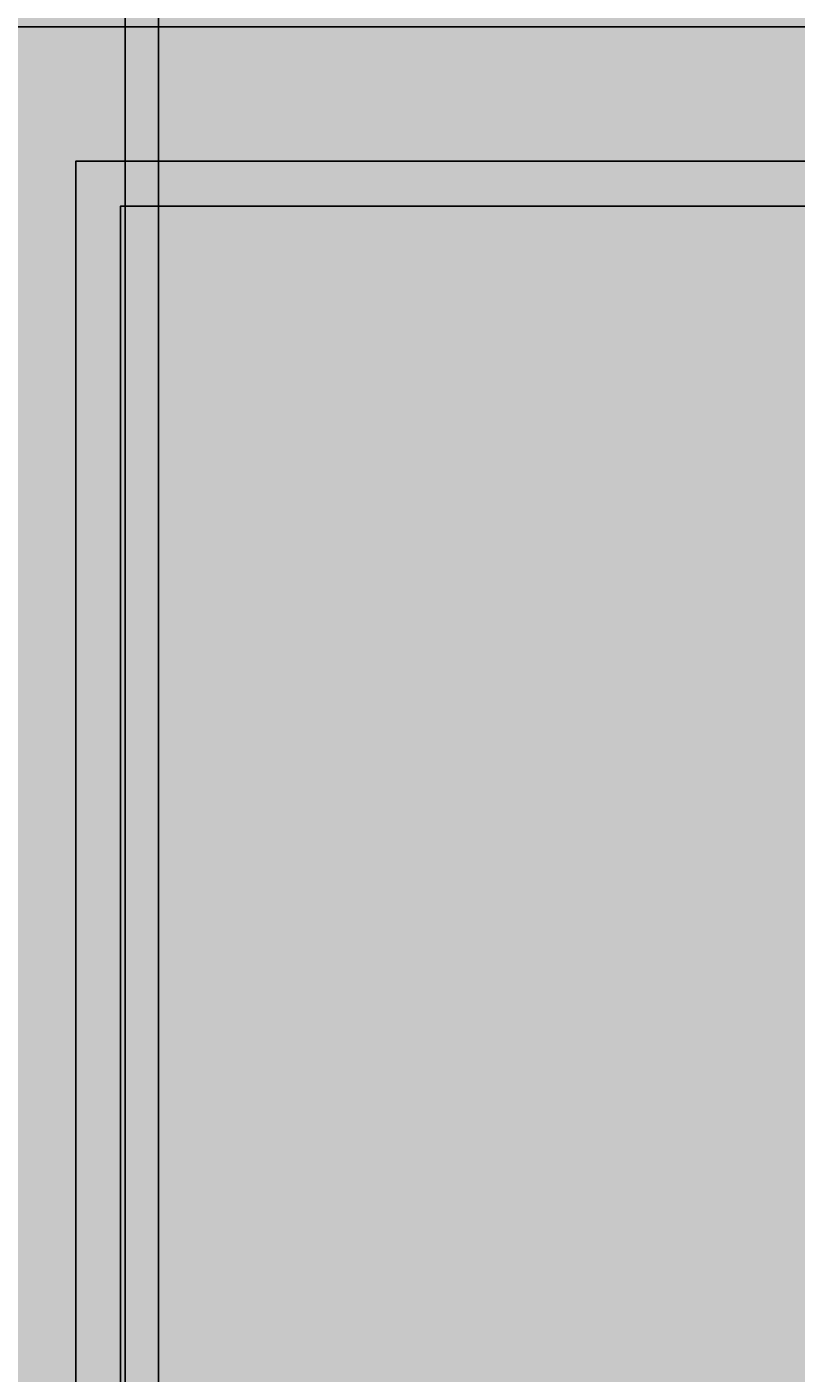
# Model space of a CAD drawing. Units: feet. Extents: x 2695 to 2912, y 795 to 1139.
# Tile 26 of 83: x 2808 to 2825, y 875 to 906. Entities that reach past the tile are written whole.
import ezdxf

# ---------------------------------------------------------------- set-up
doc = ezdxf.new("R2010")
doc.units = ezdxf.units.FT
for name, color, linetype, lineweight in [('A-ANNO-DIMS', 2, 'Continuous', 18), ('A-DOOR', 3, 'Continuous', 25), ('A-DOOR-PATT', 33, 'Continuous', 13), ('A-ELEV-PATT', 252, 'Continuous', 13)]:
    doc.layers.add(name, color=color, linetype=linetype, lineweight=lineweight)
doc.styles.get("Standard").update_dxf_attribs({"font": 'arial.ttf'})
doc.dimstyles.get("Standard").update_dxf_attribs({"dimtxt": 0.18, "dimasz": 0.18, "dimexe": 0.18, "dimexo": 0.0625, "dimgap": 0.09, "dimtad": 0, "dimtih": 1, "dimtoh": 1, "dimdec": 1, "dimzin": 0, "dimdsep": 46, "dimlunit": 3, "dimtxsty": 'Standard', "dimcen": 0.09, "dimadec": 0, "dimazin": 0, "dimtfac": 1, "dimtdec": 1, "dimtofl": 0, "dimtmove": 0, "dimatfit": 3, "dimfxl": 1, "dimtolj": 1, "dimtzin": 0, "dimarcsym": 0})

# ---------------------------------------------------------------- blocks, each defined once
blk = doc.blocks.new('*D14')
at = {"layer": 'A-ANNO-DIMS', "color": 0, "lineweight": -2, "transparency": 16777216}
for p, q in [((2838.439, 905.514), (2911.424, 905.514)), ((2911.244, 905.334), (2911.244, 890.368)), ((2911.244, 875.037), (2911.244, 890.004)), ((2758.214, 874.857), (2911.424, 874.857))]:
    blk.add_line(p, q, dxfattribs=at)
at = {"layer": 'A-ANNO-DIMS', "color": 0, "transparency": 16777216}
for points in [[(2911.214, 905.334), (2911.274, 905.334), (2911.244, 905.514)], [(2911.214, 875.037), (2911.274, 875.037), (2911.244, 874.857)]]:
    blk.add_solid(points, dxfattribs=at)
at = {"layer": 'Defpoints', "color": 0, "transparency": 16777216}
for p in [(2838.377, 905.514), (2911.244, 905.514), (2758.151, 874.857)]:
    blk.add_point(p, dxfattribs=at)
at = {"layer": 'A-ANNO-DIMS', "color": 0, "transparency": 16777216, "insert": (2911.244, 890.186), "char_height": 0.18, "attachment_point": 5}
blk.add_mtext('\\A1;30.66', dxfattribs=at)
blk = doc.blocks.new('*D52')
at = {"layer": 'A-ANNO-DIMS', "color": 0, "lineweight": -2, "transparency": 16777216}
for p, q in [((2810.041, 936.868), (2810.041, 794.976)), ((2810.789, 936.868), (2810.789, 794.976)), ((2809.861, 795.156), (2809.681, 795.156)), ((2810.969, 795.156), (2811.149, 795.156))]:
    blk.add_line(p, q, dxfattribs=at)
at = {"layer": 'A-ANNO-DIMS', "color": 0, "transparency": 16777216}
for points in [[(2809.861, 795.186), (2809.861, 795.126), (2810.041, 795.156)], [(2810.969, 795.186), (2810.969, 795.126), (2810.789, 795.156)]]:
    blk.add_solid(points, dxfattribs=at)
at = {"layer": 'Defpoints', "color": 0, "transparency": 16777216}
for p in [(2810.041, 936.931), (2810.789, 936.931), (2810.789, 795.156)]:
    blk.add_point(p, dxfattribs=at)
at = {"layer": 'A-ANNO-DIMS', "color": 0, "transparency": 16777216, "insert": (2810.415, 795.156), "char_height": 0.18, "attachment_point": 5}
blk.add_mtext('\\A1;0.75', dxfattribs=at)

msp = doc.modelspace()

# ---------------------------------------------------------------- hatches: boundary and pattern name
at = {"layer": 'A-DOOR-PATT'}
h = msp.add_hatch(color=256, dxfattribs=at)
h.set_gradient(color1=(211, 185, 150), color2=(211, 185, 150))
h.paths.add_polyline_path([(2805.9398, 905.5143), (2773.5029, 905.5143), (2773.5029, 810.9306), (2776.4999, 810.9306), (2776.4999, 902.5174), (2802.9429, 902.5174), (2802.9429, 810.9306), (2805.9398, 810.9306)])
h.paths.add_polyline_path([(2803.9681, 874.1057), (2805.0538, 874.1057), (2805.0538, 846.2857), (2803.9681, 846.2857)], flags=16)
h.paths.add_polyline_path([(2838.3767, 905.5143), (2805.9398, 905.5143), (2805.9398, 810.9306), (2808.9368, 810.9306), (2808.9368, 902.5174), (2835.3798, 902.5174), (2835.3798, 810.9306), (2838.3767, 810.9306)])
h = msp.add_hatch(color=256, dxfattribs=at)
h.set_gradient(color1=(211, 185, 150), color2=(211, 185, 150))
h.paths.add_polyline_path([(2777.5029, 901.5143), (2801.9398, 901.5143), (2801.9398, 810.9306), (2802.9429, 810.9306), (2802.9429, 902.5174), (2776.4999, 902.5174), (2776.4999, 810.9306), (2777.5029, 810.9306)])
h.paths.add_polyline_path([(2809.9398, 901.5143), (2834.3767, 901.5143), (2834.3767, 810.9306), (2835.3798, 810.9306), (2835.3798, 902.5174), (2808.9368, 902.5174), (2808.9368, 810.9306), (2809.9398, 810.9306)])
h = msp.add_hatch(color=256, dxfattribs=at)
h.set_gradient(color1=(173, 221, 247), color2=(173, 221, 247))
h.paths.add_polyline_path([(2801.9398, 901.5143), (2777.5029, 901.5143), (2777.5029, 810.9306), (2801.9398, 810.9306)])
h.paths.add_polyline_path([(2834.3767, 901.5143), (2809.9398, 901.5143), (2809.9398, 810.9306), (2834.3767, 810.9306)])
at = {"layer": 'A-ELEV-PATT'}
h = msp.add_hatch(color=256, dxfattribs=at)
h.set_gradient(color1=(147, 149, 152), color2=(147, 149, 152), tint=1)
h.paths.add_polyline_path([(2770.6361, 1118.4096), (2710.6361, 1118.4096), (2710.6361, 1062.9306), (2770.6361, 1062.9306)])
h.paths.add_polyline_path([(2890.6361, 1103.3378), (2770.6361, 1103.3378), (2770.6361, 1062.9306), (2890.6361, 1062.9306)])
h.paths.add_polyline_path([(2730.7081, 1048.1052), (2755.1125, 1048.1052), (2755.1125, 936.9306), (2770.6361, 936.9306), (2770.6361, 1050.3105), (2715.8852, 1050.3105), (2715.8852, 936.9306), (2730.7081, 936.9306)])
h.paths.add_polyline_path([(2890.6361, 1050.3105), (2770.6361, 1050.3105), (2770.6361, 971.9673), (2778.0341, 971.9673), (2778.0341, 1020.8235), (2843.575, 1020.8235), (2843.575, 971.9673), (2890.6361, 971.9673)])
h.paths.add_polyline_path([(2888.1882, 970.7156), (2843.575, 970.7156), (2843.575, 964.8267), (2888.1882, 964.8267)])
h.paths.add_polyline_path([(2888.1882, 964.1328), (2843.575, 964.1328), (2843.575, 956.614), (2888.1882, 956.614)])
h.paths.add_polyline_path([(2888.1882, 955.9202), (2843.575, 955.9202), (2843.575, 949.2892), (2888.1882, 949.2892)])
h.paths.add_polyline_path([(2888.1882, 948.5954), (2843.575, 948.5954), (2843.575, 941.3507), (2888.1882, 941.3507)])
h.paths.add_polyline_path([(2888.1882, 940.6569), (2843.575, 940.6569), (2843.575, 936.9306), (2888.1882, 936.9306)])
h.paths.add_polyline_path([(2890.6361, 970.7156), (2888.9368, 970.7156), (2888.9368, 964.8267), (2890.6361, 964.8267)])
h.paths.add_polyline_path([(2890.6361, 964.1328), (2888.9368, 964.1328), (2888.9368, 956.614), (2890.6361, 956.614)])
h.paths.add_polyline_path([(2890.6361, 955.9202), (2888.9368, 955.9202), (2888.9368, 949.2892), (2890.6361, 949.2892)])
h.paths.add_polyline_path([(2890.6361, 940.6569), (2888.9368, 940.6569), (2888.9368, 936.9306), (2890.6361, 936.9306)])
h.paths.add_polyline_path([(2890.6361, 948.5954), (2888.9368, 948.5954), (2888.9368, 941.3507), (2890.6361, 941.3507)])
h.paths.add_polyline_path([(2772.5216, 970.7156), (2770.6361, 970.7156), (2770.6361, 964.8267), (2772.5216, 964.8267)])
h.paths.add_polyline_path([(2772.5216, 964.1328), (2770.6361, 964.1328), (2770.6361, 956.614), (2772.5216, 956.614)])
h.paths.add_polyline_path([(2772.5216, 955.9202), (2770.6361, 955.9202), (2770.6361, 949.2892), (2772.5216, 949.2892)])
h.paths.add_polyline_path([(2772.5216, 948.5954), (2770.6361, 948.5954), (2770.6361, 941.3507), (2772.5216, 941.3507)])
h.paths.add_polyline_path([(2772.5216, 940.6569), (2770.6361, 940.6569), (2770.6361, 936.9306), (2772.5216, 936.9306)])
h.paths.add_polyline_path([(2778.0341, 940.6569), (2773.2702, 940.6569), (2773.2702, 936.9306), (2778.0341, 936.9306)])
h.paths.add_polyline_path([(2778.0341, 970.7156), (2773.2702, 970.7156), (2773.2702, 964.8267), (2778.0341, 964.8267)])
h.paths.add_polyline_path([(2778.0341, 964.1328), (2773.2702, 964.1328), (2773.2702, 956.614), (2778.0341, 956.614)])
h.paths.add_polyline_path([(2778.0341, 955.9202), (2773.2702, 955.9202), (2773.2702, 949.2892), (2778.0341, 949.2892)])
h.paths.add_polyline_path([(2778.0341, 948.5954), (2773.2702, 948.5954), (2773.2702, 941.3507), (2778.0341, 941.3507)])
h.paths.add_polyline_path([(2810.0407, 940.6569), (2780.0341, 940.6569), (2780.0341, 936.9306), (2810.0407, 936.9306)])
h.paths.add_polyline_path([(2890.6361, 924.3105), (2770.6361, 924.3105), (2770.6361, 810.9306), (2773.5029, 810.9306), (2773.5029, 905.5143), (2805.9398, 905.5143), (2838.3767, 905.5143), (2838.3767, 810.9306), (2890.6361, 810.9306)])

# ---------------------------------------------------------------- linework, layer by layer
at = {"layer": 'A-DOOR'}
for points in [[(2773.5029, 905.5143), (2838.3767, 905.5143), (2838.3767, 810.9306), (2773.5029, 810.9306)], [(2808.9368, 902.5174), (2835.3798, 902.5174), (2835.3798, 810.9306), (2808.9368, 810.9306)], [(2809.9398, 901.5143), (2834.3767, 901.5143), (2834.3767, 810.9306), (2809.9398, 810.9306)]]:
    msp.add_lwpolyline(points, close=True, dxfattribs=at)
for points in [[(2838.3767, 810.9306), (2838.3767, 905.5143), (2805.9398, 905.5143), (2805.9398, 810.9306)], [(2835.3798, 810.9306), (2835.3798, 902.5174), (2808.9368, 902.5174), (2808.9368, 810.9306)], [(2834.3767, 810.9306), (2834.3767, 901.5143), (2809.9398, 901.5143), (2809.9398, 810.9306)]]:
    msp.add_lwpolyline(points, dxfattribs=at)

# ---------------------------------------------------------------- dimensions: what is measured, and where the dimension line sits
at = {"layer": 'A-ANNO-DIMS'}
dim = msp.add_linear_dim(base=(2810.7893, 795.1556), p1=(2810.0407, 936.9306), p2=(2810.7893, 936.9306), dimstyle='Standard', override={"dimdec": 2, "dimlfac": 1, "dimrnd": 0, "dimzin": 0, "dimdsep": 46, "dimlunit": 2}, dxfattribs=at)
dim.commit()
dim.dimension.update_dxf_attribs({"geometry": '*D52', "text_midpoint": (2810.415, 795.1556)})
dim = msp.add_linear_dim(base=(2911.2444, 905.5143), p1=(2758.1515, 874.8571), p2=(2838.3767, 905.5143), angle=90, dimstyle='Standard', override={"dimdec": 2, "dimlfac": 1, "dimrnd": 0, "dimzin": 0, "dimdsep": 46, "dimlunit": 2}, dxfattribs=at)
dim.commit()
dim.dimension.update_dxf_attribs({"geometry": '*D14', "text_midpoint": (2911.2444, 890.1857)})

doc.saveas('drawing.dxf')
